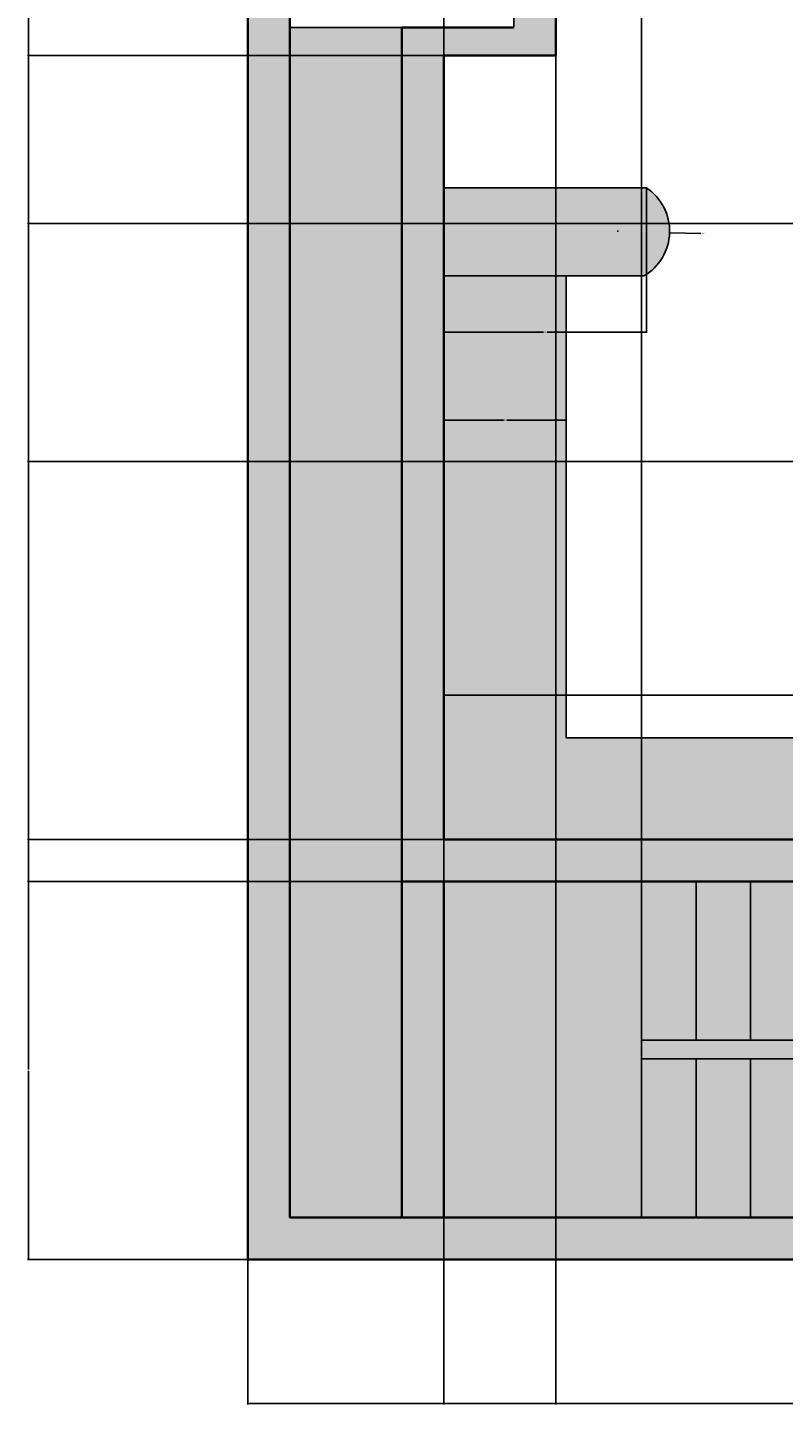
# Model space of a CAD drawing. Units: inches. Extents: x 2549 to 3108, y 1683 to 2362.
# Tile 1 of 30: x 2549 to 2711, y 1683 to 1979. Entities that reach past the tile are written whole.
import ezdxf

# ---------------------------------------------------------------- set-up
doc = ezdxf.new("R2010")
doc.units = ezdxf.units.IN
for name, color, linetype, lineweight in [('A-ANNO-DIMS', 2, 'Continuous', 18), ('A-FLOR', 7, 'Continuous', 25), ('A-FLOR-CASE', 8, 'Continuous', 25), ('A-FLOR-CASE-PATT', 42, 'Continuous', 13), ('A-FLOR-STRS', 7, 'Continuous', 25), ('A-FLOR-STRS-PATT', 41, 'Continuous', 13), ('A-WALL', 7, 'Continuous', 35), ('A-WALL-PATT', 89, 'Continuous', 13), ('C-PROP', 7, 'Continuous', 35)]:
    doc.layers.add(name, color=color, linetype=linetype, lineweight=lineweight)
for name, color, linetype, lineweight, true_color in [('C-PKNG-VEHI-PATT', 251, 'Continuous', 13, 0x636466), ('C-PROP-PATT', 252, 'Continuous', 13, 0x939598), ('C-PVMT-PATT', 9, 'Continuous', 13, 0xc7c8ca)]:
    doc.layers.add(name, color=color, linetype=linetype, lineweight=lineweight, true_color=true_color)
doc.styles.get("Standard").update_dxf_attribs({"font": 'arial.ttf'})
doc.dimstyles.get("Standard").update_dxf_attribs({"dimtxt": 0.18, "dimasz": 0.18, "dimexe": 0.18, "dimexo": 0.0625, "dimgap": 0.09, "dimtad": 0, "dimtih": 1, "dimtoh": 1, "dimdec": 4, "dimzin": 0, "dimdsep": 46, "dimtxsty": 'Standard', "dimcen": 0.09, "dimadec": 0, "dimazin": 0, "dimtfac": 1, "dimtdec": 4, "dimtofl": 0, "dimtmove": 0, "dimatfit": 3, "dimfxl": 1, "dimtolj": 1, "dimtzin": 0, "dimarcsym": 0})

# ---------------------------------------------------------------- blocks, each defined once
blk = doc.blocks.new('*D24')
at = {"layer": 'A-ANNO-DIMS', "color": 0, "lineweight": -2, "transparency": 16777216}
for p, q in [((2596.64, 1714.46), (2596.64, 1683.44)), ((3076.64, 1714.46), (3076.64, 1683.44)), ((2596.82, 1683.62), (2836.35, 1683.62)), ((3076.46, 1683.62), (2836.93, 1683.62))]:
    blk.add_line(p, q, dxfattribs=at)
at = {"layer": 'A-ANNO-DIMS', "color": 0, "transparency": 16777216}
for points in [[(2596.82, 1683.65), (2596.82, 1683.59), (2596.64, 1683.62)], [(3076.46, 1683.65), (3076.46, 1683.59), (3076.64, 1683.62)]]:
    blk.add_solid(points, dxfattribs=at)
at = {"layer": 'Defpoints', "color": 0, "transparency": 16777216}
for p in [(2596.64, 1714.52), (3076.64, 1714.52), (3076.64, 1683.62)]:
    blk.add_point(p, dxfattribs=at)
at = {"layer": 'A-ANNO-DIMS', "color": 0, "transparency": 16777216, "insert": (2836.64, 1683.62), "char_height": 0.18, "attachment_point": 5}
blk.add_mtext('\\A1;480', dxfattribs=at)
blk = doc.blocks.new('*D34')
at = {"layer": 'A-ANNO-DIMS', "color": 0, "lineweight": -2, "transparency": 16777216}
for p, q in [((2629.58, 2074.52), (2549.42, 2074.52)), ((2549.6, 2074.34), (2549.6, 2023.71)), ((2549.6, 1972.7), (2549.6, 2023.34)), ((2638.58, 1972.52), (2549.42, 1972.52))]:
    blk.add_line(p, q, dxfattribs=at)
at = {"layer": 'A-ANNO-DIMS', "color": 0, "transparency": 16777216}
for points in [[(2549.57, 2074.34), (2549.63, 2074.34), (2549.6, 2074.52)], [(2549.57, 1972.7), (2549.63, 1972.7), (2549.6, 1972.52)]]:
    blk.add_solid(points, dxfattribs=at)
at = {"layer": 'Defpoints', "color": 0, "transparency": 16777216}
for p in [(2549.6, 2074.52), (2629.64, 2074.52), (2638.64, 1972.52)]:
    blk.add_point(p, dxfattribs=at)
at = {"layer": 'A-ANNO-DIMS', "color": 0, "transparency": 16777216, "insert": (2549.6, 2023.52), "char_height": 0.18, "attachment_point": 5}
blk.add_mtext('\\A1;102', dxfattribs=at)
blk = doc.blocks.new('*D35')
at = {"layer": 'A-ANNO-DIMS', "color": 0, "lineweight": -2, "transparency": 16777216}
for p, q in [((2638.58, 1972.52), (2549.42, 1972.52)), ((2549.6, 1972.34), (2549.6, 1884.2)), ((2549.6, 1795.7), (2549.6, 1883.84)), ((2629.58, 1795.52), (2549.42, 1795.52))]:
    blk.add_line(p, q, dxfattribs=at)
at = {"layer": 'A-ANNO-DIMS', "color": 0, "transparency": 16777216}
for points in [[(2549.57, 1972.34), (2549.63, 1972.34), (2549.6, 1972.52)], [(2549.57, 1795.7), (2549.63, 1795.7), (2549.6, 1795.52)]]:
    blk.add_solid(points, dxfattribs=at)
at = {"layer": 'Defpoints', "color": 0, "transparency": 16777216}
for p in [(2549.6, 1972.52), (2638.64, 1972.52), (2629.64, 1795.52)]:
    blk.add_point(p, dxfattribs=at)
at = {"layer": 'A-ANNO-DIMS', "color": 0, "transparency": 16777216, "insert": (2549.6, 1884.02), "char_height": 0.18, "attachment_point": 5}
blk.add_mtext('\\A1;177', dxfattribs=at)
blk = doc.blocks.new('*D36')
at = {"layer": 'A-ANNO-DIMS', "color": 0, "lineweight": -2, "transparency": 16777216}
for p, q in [((2629.58, 1795.52), (2549.42, 1795.52)), ((2549.6, 1795.34), (2549.6, 1755.21)), ((2549.6, 1714.7), (2549.6, 1754.84)), ((2596.58, 1714.52), (2549.42, 1714.52))]:
    blk.add_line(p, q, dxfattribs=at)
at = {"layer": 'A-ANNO-DIMS', "color": 0, "transparency": 16777216}
for points in [[(2549.57, 1795.34), (2549.63, 1795.34), (2549.6, 1795.52)], [(2549.57, 1714.7), (2549.63, 1714.7), (2549.6, 1714.52)]]:
    blk.add_solid(points, dxfattribs=at)
at = {"layer": 'Defpoints', "color": 0, "transparency": 16777216}
for p in [(2549.6, 1795.52), (2629.64, 1795.52), (2596.64, 1714.52)]:
    blk.add_point(p, dxfattribs=at)
at = {"layer": 'A-ANNO-DIMS', "color": 0, "transparency": 16777216, "insert": (2549.6, 1755.02), "char_height": 0.18, "attachment_point": 5}
blk.add_mtext('\\A1;81', dxfattribs=at)
blk = doc.blocks.new('*D42')
at = {"layer": 'A-ANNO-DIMS', "color": 0, "lineweight": -2, "transparency": 16777216}
for p, q in [((2638.64, 2080.46), (2638.64, 1683.44)), ((2728.64, 2080.46), (2728.64, 1683.44)), ((2638.82, 1683.62), (2683.42, 1683.62)), ((2728.46, 1683.62), (2683.86, 1683.62))]:
    blk.add_line(p, q, dxfattribs=at)
at = {"layer": 'A-ANNO-DIMS', "color": 0, "transparency": 16777216}
for points in [[(2638.82, 1683.65), (2638.82, 1683.59), (2638.64, 1683.62)], [(2728.46, 1683.65), (2728.46, 1683.59), (2728.64, 1683.62)]]:
    blk.add_solid(points, dxfattribs=at)
at = {"layer": 'Defpoints', "color": 0, "transparency": 16777216}
for p in [(2638.64, 2080.52), (2728.64, 2080.52), (2728.64, 1683.62)]:
    blk.add_point(p, dxfattribs=at)
at = {"layer": 'A-ANNO-DIMS', "color": 0, "transparency": 16777216, "insert": (2683.64, 1683.62), "char_height": 0.18, "attachment_point": 5}
blk.add_mtext('\\A1;90', dxfattribs=at)
blk = doc.blocks.new('*D44')
at = {"layer": 'A-ANNO-DIMS', "color": 0, "lineweight": -2, "transparency": 16777216}
for p, q in [((2662.64, 2040.99), (2662.64, 1683.44)), ((2806.64, 2016.13), (2806.64, 1683.44)), ((2662.82, 1683.62), (2734.36, 1683.62)), ((2806.46, 1683.62), (2734.92, 1683.62))]:
    blk.add_line(p, q, dxfattribs=at)
at = {"layer": 'A-ANNO-DIMS', "color": 0, "transparency": 16777216}
for points in [[(2662.82, 1683.65), (2662.82, 1683.59), (2662.64, 1683.62)], [(2806.46, 1683.65), (2806.46, 1683.59), (2806.64, 1683.62)]]:
    blk.add_solid(points, dxfattribs=at)
at = {"layer": 'Defpoints', "color": 0, "transparency": 16777216}
for p in [(2662.64, 2041.06), (2806.64, 2016.19), (2806.64, 1683.62)]:
    blk.add_point(p, dxfattribs=at)
at = {"layer": 'A-ANNO-DIMS', "color": 0, "transparency": 16777216, "insert": (2734.64, 1683.62), "char_height": 0.18, "attachment_point": 5}
blk.add_mtext('\\A1;144', dxfattribs=at)
blk = doc.blocks.new('*D45')
at = {"layer": 'A-ANNO-DIMS', "color": 0, "lineweight": -2, "transparency": 16777216}
for p, q in [((2605.64, 1978.59), (2605.64, 2009.6)), ((2653.64, 1978.59), (2653.64, 2009.6)), ((2605.82, 2009.42), (2629.42, 2009.42)), ((2653.46, 2009.42), (2629.87, 2009.42))]:
    blk.add_line(p, q, dxfattribs=at)
at = {"layer": 'A-ANNO-DIMS', "color": 0, "transparency": 16777216}
for points in [[(2605.82, 2009.45), (2605.82, 2009.39), (2605.64, 2009.42)], [(2653.46, 2009.45), (2653.46, 2009.39), (2653.64, 2009.42)]]:
    blk.add_solid(points, dxfattribs=at)
at = {"layer": 'Defpoints', "color": 0, "transparency": 16777216}
for p in [(2653.64, 2009.42), (2605.64, 1978.52), (2653.64, 1978.52)]:
    blk.add_point(p, dxfattribs=at)
at = {"layer": 'A-ANNO-DIMS', "color": 0, "transparency": 16777216, "insert": (2629.64, 2009.42), "char_height": 0.18, "attachment_point": 5}
blk.add_mtext('\\A1;48', dxfattribs=at)
blk = doc.blocks.new('*D49')
at = {"layer": 'A-ANNO-DIMS', "color": 0, "lineweight": -2, "transparency": 16777216}
for p, q in [((2638.64, 1804.59), (2638.64, 1835.6)), ((2638.82, 1835.42), (2722.36, 1835.42)), ((2806.46, 1835.42), (2722.92, 1835.42)), ((2806.64, 1804.59), (2806.64, 1835.6))]:
    blk.add_line(p, q, dxfattribs=at)
at = {"layer": 'A-ANNO-DIMS', "color": 0, "transparency": 16777216}
for points in [[(2638.82, 1835.45), (2638.82, 1835.39), (2638.64, 1835.42)], [(2806.46, 1835.45), (2806.46, 1835.39), (2806.64, 1835.42)]]:
    blk.add_solid(points, dxfattribs=at)
at = {"layer": 'Defpoints', "color": 0, "transparency": 16777216}
for p in [(2806.64, 1835.42), (2638.64, 1804.52), (2806.64, 1804.52)]:
    blk.add_point(p, dxfattribs=at)
at = {"layer": 'A-ANNO-DIMS', "color": 0, "transparency": 16777216, "insert": (2722.64, 1835.42), "char_height": 0.18, "attachment_point": 5}
blk.add_mtext('\\A1;168', dxfattribs=at)
blk = doc.blocks.new('*D50')
at = {"layer": 'A-ANNO-DIMS', "color": 0, "lineweight": -2, "transparency": 16777216}
for p, q in [((2638.64, 1944.09), (2638.64, 1913.07)), ((2682.05, 1944.09), (2682.05, 1913.07)), ((2638.82, 1913.25), (2659.97, 1913.25)), ((2681.87, 1913.25), (2660.73, 1913.25))]:
    blk.add_line(p, q, dxfattribs=at)
at = {"layer": 'A-ANNO-DIMS', "color": 0, "transparency": 16777216}
for points in [[(2638.82, 1913.28), (2638.82, 1913.22), (2638.64, 1913.25)], [(2681.87, 1913.28), (2681.87, 1913.22), (2682.05, 1913.25)]]:
    blk.add_solid(points, dxfattribs=at)
at = {"layer": 'Defpoints', "color": 0, "transparency": 16777216}
for p in [(2638.64, 1944.15), (2682.05, 1944.15), (2638.64, 1913.25)]:
    blk.add_point(p, dxfattribs=at)
at = {"layer": 'A-ANNO-DIMS', "color": 0, "transparency": 16777216, "insert": (2660.35, 1913.25), "char_height": 0.18, "attachment_point": 5}
blk.add_mtext('\\A1;43.41', dxfattribs=at)
blk = doc.blocks.new('*D51')
at = {"layer": 'A-ANNO-DIMS', "color": 0, "lineweight": -2, "transparency": 16777216}
for p, q in [((2638.64, 1925.23), (2638.64, 1894.21)), ((2664.85, 1925.23), (2664.85, 1894.21)), ((2638.82, 1894.39), (2651.37, 1894.39)), ((2664.67, 1894.39), (2652.13, 1894.39))]:
    blk.add_line(p, q, dxfattribs=at)
at = {"layer": 'A-ANNO-DIMS', "color": 0, "transparency": 16777216}
for points in [[(2638.82, 1894.42), (2638.82, 1894.36), (2638.64, 1894.39)], [(2664.67, 1894.42), (2664.67, 1894.36), (2664.85, 1894.39)]]:
    blk.add_solid(points, dxfattribs=at)
at = {"layer": 'Defpoints', "color": 0, "transparency": 16777216}
for p in [(2638.64, 1925.29), (2664.85, 1925.29), (2638.64, 1894.39)]:
    blk.add_point(p, dxfattribs=at)
at = {"layer": 'A-ANNO-DIMS', "color": 0, "transparency": 16777216, "insert": (2651.75, 1894.39), "char_height": 0.18, "attachment_point": 5}
blk.add_mtext('\\A1;26.21', dxfattribs=at)
blk = doc.blocks.new('*D55')
at = {"layer": 'A-ANNO-DIMS', "color": 0, "lineweight": -2, "transparency": 16777216}
for p, q in [((2872.58, 1885.52), (2549.42, 1885.52)), ((2549.6, 1885.34), (2549.6, 1845.21)), ((2549.6, 1804.7), (2549.6, 1844.84)), ((2872.58, 1804.52), (2549.42, 1804.52))]:
    blk.add_line(p, q, dxfattribs=at)
at = {"layer": 'A-ANNO-DIMS', "color": 0, "transparency": 16777216}
for points in [[(2549.57, 1885.34), (2549.63, 1885.34), (2549.6, 1885.52)], [(2549.57, 1804.7), (2549.63, 1804.7), (2549.6, 1804.52)]]:
    blk.add_solid(points, dxfattribs=at)
at = {"layer": 'Defpoints', "color": 0, "transparency": 16777216}
for p in [(2549.6, 1885.52), (2872.64, 1885.52), (2872.64, 1804.52)]:
    blk.add_point(p, dxfattribs=at)
at = {"layer": 'A-ANNO-DIMS', "color": 0, "transparency": 16777216, "insert": (2549.6, 1845.02), "char_height": 0.18, "attachment_point": 5}
blk.add_mtext('\\A1;81', dxfattribs=at)
blk = doc.blocks.new('*D56')
at = {"layer": 'A-ANNO-DIMS', "color": 0, "lineweight": -2, "transparency": 16777216}
for p, q in [((3043.58, 1936.52), (2549.42, 1936.52)), ((2549.6, 1936.34), (2549.6, 1911.21)), ((2549.6, 1885.7), (2549.6, 1910.84)), ((3043.58, 1885.52), (2549.42, 1885.52))]:
    blk.add_line(p, q, dxfattribs=at)
at = {"layer": 'A-ANNO-DIMS', "color": 0, "transparency": 16777216}
for points in [[(2549.57, 1936.34), (2549.63, 1936.34), (2549.6, 1936.52)], [(2549.57, 1885.7), (2549.63, 1885.7), (2549.6, 1885.52)]]:
    blk.add_solid(points, dxfattribs=at)
at = {"layer": 'Defpoints', "color": 0, "transparency": 16777216}
for p in [(2549.6, 1936.52), (3043.64, 1936.52), (3043.64, 1885.52)]:
    blk.add_point(p, dxfattribs=at)
at = {"layer": 'A-ANNO-DIMS', "color": 0, "transparency": 16777216, "insert": (2549.6, 1911.02), "char_height": 0.18, "attachment_point": 5}
blk.add_mtext('\\A1;51', dxfattribs=at)
blk = doc.blocks.new('*D59')
at = {"layer": 'A-ANNO-DIMS', "color": 0, "lineweight": -2, "transparency": 16777216}
for p, q in [((2680.98, 1761.59), (2680.98, 2362.32)), ((2681.16, 2362.14), (2733.11, 2362.14)), ((2785.98, 2362.14), (2734.02, 2362.14)), ((2786.16, 1761.59), (2786.16, 2362.32))]:
    blk.add_line(p, q, dxfattribs=at)
at = {"layer": 'A-ANNO-DIMS', "color": 0, "transparency": 16777216}
for points in [[(2681.16, 2362.17), (2681.16, 2362.11), (2680.98, 2362.14)], [(2785.98, 2362.17), (2785.98, 2362.11), (2786.16, 2362.14)]]:
    blk.add_solid(points, dxfattribs=at)
at = {"layer": 'Defpoints', "color": 0, "transparency": 16777216}
for p in [(2786.16, 2362.14), (2680.98, 1761.52), (2786.16, 1761.52)]:
    blk.add_point(p, dxfattribs=at)
at = {"layer": 'A-ANNO-DIMS', "color": 0, "transparency": 16777216, "insert": (2733.57, 2362.14), "char_height": 0.18, "attachment_point": 5}
blk.add_mtext('\\A1;105.18', dxfattribs=at)
blk = doc.blocks.new('*D62')
at = {"layer": 'A-ANNO-DIMS', "color": 0, "lineweight": -2, "transparency": 16777216}
for p, q in [((2675.78, 1934.89), (2675.96, 1934.89)), ((2675.87, 1934.8), (2675.87, 1934.98)), ((2693.67, 1934.38), (2687.18, 1934.56))]:
    blk.add_line(p, q, dxfattribs=at)
at = {"layer": 'A-ANNO-DIMS', "color": 0, "transparency": 16777216}
blk.add_solid([(2687.18, 1934.59), (2687.18, 1934.53), (2687, 1934.57)], dxfattribs=at)
at = {"layer": 'Defpoints', "color": 0, "transparency": 16777216}
for p in [(2675.87, 1934.89), (2687, 1934.57)]:
    blk.add_point(p, dxfattribs=at)
at = {"layer": 'A-ANNO-DIMS', "color": 0, "transparency": 16777216, "insert": (2694.15, 1934.38), "char_height": 0.18, "attachment_point": 5}
blk.add_mtext('\\A1;R11.13', dxfattribs=at)

msp = doc.modelspace()

# ---------------------------------------------------------------- hatches: boundary and pattern name
at = {"layer": 'A-FLOR-CASE-PATT', "transparency": 33554595}
h = msp.add_hatch(color=256, dxfattribs=at)
h.dxf.hatch_style = 1
h.paths.add_polyline_path([(2682.0533, 1944.149), (2638.6427, 1944.149), (2638.6427, 1925.2912), (2681.5046, 1925.2912, 0.55362962)])
at = {"layer": 'A-FLOR-CASE-PATT', "transparency": 33554539}
h = msp.add_hatch(color=256, dxfattribs=at)
h.dxf.hatch_style = 1
h.paths.add_polyline_path([(2664.8522, 1925.2912), (2638.6427, 1925.2912), (2638.6427, 1804.5237), (2662.6427, 1804.5237), (2806.6427, 1804.5237), (2806.6427, 1826.2821), (2664.8522, 1826.2821)])
h.paths.add_polyline_path([(2872.6427, 1885.5237), (2858.0172, 1885.5237), (2858.0172, 1818.9517), (2812.6427, 1818.9517), (2812.6427, 1804.5237), (2872.6427, 1804.5237)])
at = {"layer": 'A-FLOR-STRS-PATT', "transparency": 33554567}
h = msp.add_hatch(color=256, dxfattribs=at)
h.dxf.hatch_style = 1
h.paths.add_polyline_path([(2680.9778, 1795.5237), (2662.6427, 1795.5237), (2638.6427, 1795.5237), (2638.6427, 1723.5237), (2680.9778, 1723.5237)])
h.paths.add_polyline_path([(2692.6645, 1795.5237), (2680.9778, 1795.5237), (2680.9778, 1761.5237), (2692.6645, 1761.5237)])
h.paths.add_polyline_path([(2704.3511, 1795.5237), (2692.6645, 1795.5237), (2692.6645, 1761.5237), (2704.3511, 1761.5237)])
h.paths.add_polyline_path([(2716.0378, 1795.5237), (2704.3511, 1795.5237), (2704.3511, 1761.5237), (2716.0378, 1761.5237)])
h.paths.add_polyline_path([(2727.7244, 1795.5237), (2716.0378, 1795.5237), (2716.0378, 1761.5237), (2727.7244, 1761.5237)])
h.paths.add_polyline_path([(2739.4111, 1795.5237), (2727.7244, 1795.5237), (2727.7244, 1761.5237), (2739.4111, 1761.5237)])
h.paths.add_polyline_path([(2751.0977, 1795.5237), (2739.4111, 1795.5237), (2739.4111, 1761.5237), (2751.0977, 1761.5237)])
h.paths.add_polyline_path([(2786.1577, 1757.5237), (2774.471, 1757.5237), (2774.471, 1723.5237), (2786.1577, 1723.5237)])
h.paths.add_polyline_path([(2774.471, 1757.5237), (2762.7844, 1757.5237), (2762.7844, 1723.5237), (2774.471, 1723.5237)])
h.paths.add_polyline_path([(2762.7844, 1757.5237), (2751.0977, 1757.5237), (2751.0977, 1723.5237), (2762.7844, 1723.5237)])
h.paths.add_polyline_path([(2751.0977, 1757.5237), (2739.4111, 1757.5237), (2739.4111, 1723.5237), (2751.0977, 1723.5237)])
h.paths.add_polyline_path([(2727.7244, 1757.5237), (2716.0378, 1757.5237), (2716.0378, 1723.5237), (2727.7244, 1723.5237)])
h.paths.add_polyline_path([(2716.0378, 1757.5237), (2704.3511, 1757.5237), (2704.3511, 1723.5237), (2716.0378, 1723.5237)])
h.paths.add_polyline_path([(2704.3511, 1757.5237), (2692.6645, 1757.5237), (2692.6645, 1723.5237), (2704.3511, 1723.5237)])
h.paths.add_polyline_path([(2692.6645, 1757.5237), (2680.9778, 1757.5237), (2680.9778, 1723.5237), (2692.6645, 1723.5237)])
h.paths.add_polyline_path([(2739.4111, 1757.5237), (2727.7244, 1757.5237), (2727.7244, 1723.5237), (2739.4111, 1723.5237)])
h.paths.add_polyline_path([(2786.1577, 1761.5237), (2680.9778, 1761.5237), (2680.9778, 1757.5237), (2786.1577, 1757.5237)])
at = {"layer": 'A-WALL-PATT'}
h = msp.add_hatch(color=256, dxfattribs=at)
h.dxf.hatch_style = 1
h.paths.add_polyline_path([(2638.6427, 2272.5237), (3034.6427, 2272.5237), (3034.6427, 1936.5237), (3043.6427, 1936.5237), (3043.6427, 2281.5237), (2629.6427, 2281.5237), (2629.6427, 2074.5237), (2812.6427, 2074.5237), (2812.6427, 2140.5237), (2785.7177, 2140.5237), (2785.7177, 2134.5237), (2806.6427, 2134.5237), (2806.6427, 2080.5237), (2638.6427, 2080.5237)])
h.paths.add_polyline_path([(2638.6427, 1972.5237), (2662.6427, 1972.5237), (2662.6427, 2041.0557), (2653.6427, 2041.0557), (2653.6427, 1978.5237), (2629.6427, 1978.5237), (2629.6427, 1795.5237), (2662.6427, 1795.5237), (2881.6427, 1795.5237), (2881.6427, 1936.5237), (2965.9351, 1936.5237), (2965.9351, 1974.5439), (2959.9351, 1974.5439), (2959.9351, 1945.5237), (2881.6427, 1945.5237), (2872.6427, 1945.5237), (2872.6427, 1804.5237), (2662.6427, 1804.5237), (2638.6427, 1804.5237)])
h = msp.add_hatch(color=256, dxfattribs=at)
h.dxf.hatch_style = 1
h.paths.add_polyline_path([(2638.6427, 1795.5237), (2629.6427, 1795.5237), (2629.6427, 1723.5237), (2638.6427, 1723.5237)])
at = {"layer": 'C-PKNG-VEHI-PATT'}
h = msp.add_hatch(color=256, dxfattribs=at)
h.dxf.hatch_style = 1
edge = h.paths.add_edge_path()
edge.add_ellipse((2935.7258, 1791.964), major_axis=(-50.66, 0), ratio=0.84230387, start_angle=248.165046, end_angle=265.722579)
edge.add_line((2938.911, 1834.5507), (2925.8653, 1834.5507))
edge.add_ellipse((2929.0505, 1791.964), major_axis=(50.66, 0), ratio=0.84230387, start_angle=94.277421, end_angle=111.834954)
edge.add_line((2912.8508, 1832.3947), (2914.2044, 1822.2495))
edge.add_ellipse((2930.6538, 1783.1023), major_axis=(-49.3014, 0), ratio=0.84230387, start_angle=-85.12993, end_angle=-67.208085, ccw=False)
edge.add_line((2927.1247, 1824.5225), (2937.6516, 1824.5225))
edge.add_ellipse((2934.1225, 1783.1023), major_axis=(49.3014, 0), ratio=0.84230387, start_angle=67.208085, end_angle=85.12993, ccw=False)
edge.add_line((2950.5719, 1822.2495), (2951.9255, 1832.3947))
edge = h.paths.add_edge_path()
edge.add_ellipse((2903.4793, 1857.3351), major_axis=(-34.7979, 0), ratio=0.84230387, start_angle=180, end_angle=209.43857)
edge.add_ellipse((2961.297, 1857.3351), major_axis=(34.7979, 0), ratio=0.84230387, start_angle=150.56143, end_angle=180)
edge.add_line((2926.4991, 1857.3351), (2926.4991, 1843.7609))
edge.add_ellipse((2924.1251, 1844.3143), major_axis=(-0.2209, 3.9278), ratio=0.60383358, start_angle=89.002014, end_angle=253.657408, ccw=False)
edge.add_line((2921.7512, 1844.2222), (2921.7512, 1853.3975))
edge.add_line((2921.7512, 1853.3975), (2925.269, 1855.8484))
edge.add_ellipse((2925.4782, 1855.4931), major_axis=(0.4584, 0), ratio=0.84230387, start_angle=90, end_angle=134.480211, ccw=False)
edge.add_line((2925.4782, 1855.8792), (2926.4991, 1855.8792))
edge.add_line((2926.4991, 1855.8792), (2926.4991, 1857.3351))
edge.add_ellipse((2961.297, 1857.3351), major_axis=(34.7979, 0), ratio=0.84230387, start_angle=150.56143, end_angle=180, ccw=False)
edge.add_line((2932.3882, 1873.6501), (2932.3882, 1875.7801))
edge.add_ellipse((2932.3882, 1875.3939), major_axis=(0.4584, 0), ratio=0.84230387, start_angle=90, end_angle=127.93313)
edge.add_line((2932.1366, 1875.7167), (2928.5915, 1873.7564))
edge.add_ellipse((2899.9271, 2002.4692), major_axis=(155.4756, 0), ratio=0.84230387, start_angle=-80.743434, end_angle=-77.445067, ccw=False)
edge.add_ellipse((2949.4402, 1715.2151), major_axis=(-189.1422, 0), ratio=0.84230387, start_angle=-79.790461, end_angle=-77.555373)
edge.add_ellipse((3300.3614, 1852.5642), major_axis=(-386.1662, 0), ratio=0.84230387, start_angle=-2.863715, end_angle=2.198541)
edge.add_ellipse((2929.0505, 1792.5159), major_axis=(-55.6192, 0), ratio=0.84230387, start_angle=-85.917589, end_angle=-72.280047, ccw=False)
edge.add_line((2925.7129, 1839.2798), (2939.0634, 1839.2798))
edge.add_ellipse((2935.7258, 1792.5159), major_axis=(55.6192, 0), ratio=0.84230387, start_angle=72.280047, end_angle=85.917589, ccw=False)
edge.add_ellipse((2564.4149, 1852.5642), major_axis=(-386.1662, 0), ratio=0.84230387, start_angle=177.801459, end_angle=182.863715)
edge.add_ellipse((2915.3361, 1715.2151), major_axis=(189.1422, 0), ratio=0.84230387, start_angle=77.555373, end_angle=79.790461)
edge.add_ellipse((2964.8492, 2002.4692), major_axis=(-155.4756, 0), ratio=0.84230387, start_angle=77.445067, end_angle=80.743434, ccw=False)
edge.add_line((2936.1848, 1873.7564), (2932.6397, 1875.7167))
edge.add_ellipse((2932.3882, 1875.3939), major_axis=(0.4584, 0), ratio=0.84230387, start_angle=52.06687, end_angle=90)
edge.add_line((2932.3882, 1875.7801), (2932.3882, 1873.6501))
edge.add_ellipse((2903.4793, 1857.3351), major_axis=(-34.7979, 0), ratio=0.84230387, start_angle=180, end_angle=209.43857, ccw=False)
edge.add_line((2938.2772, 1857.3351), (2938.2772, 1855.8792))
edge.add_line((2938.2772, 1855.8792), (2939.4059, 1855.8792))
edge.add_ellipse((2939.2981, 1855.4931), major_axis=(-0.4584, 0), ratio=0.84230387, start_angle=225.519789, end_angle=270, ccw=False)
edge.add_line((2939.5903, 1855.7906), (2943.0251, 1853.3975))
edge.add_line((2943.0251, 1853.3975), (2943.0251, 1844.2222))
edge.add_ellipse((2940.6512, 1844.3143), major_axis=(0.2209, 3.9278), ratio=0.60383358, start_angle=106.342592, end_angle=270.997986, ccw=False)
edge.add_line((2938.2772, 1843.7609), (2938.2772, 1857.3351))
edge = h.paths.add_edge_path()
edge.add_ellipse((2932.3882, 1865.1973), major_axis=(91.081, 0), ratio=0.84230387, start_angle=256.401865, end_angle=283.598135, ccw=False)
edge.add_line((2914.2044, 1790.0239), (2914.2044, 1778.3622))
edge.add_ellipse((2932.3882, 1853.5356), major_axis=(91.081, 0), ratio=0.84230387, start_angle=256.401865, end_angle=283.598135)
edge.add_line((2950.5719, 1778.3622), (2950.5719, 1790.0239))
edge = h.paths.add_edge_path()
edge.add_ellipse((2948.7383, 1772.3145), major_axis=(1.8336, 0), ratio=0.84230387, start_angle=0, end_angle=90)
edge.add_line((2948.7383, 1773.859), (2916.038, 1773.859))
edge.add_ellipse((2916.038, 1772.3145), major_axis=(1.8336, 0), ratio=0.84230387, start_angle=90, end_angle=180)
edge.add_line((2914.2044, 1772.3145), (2914.2044, 1760.2558))
edge.add_line((2914.2044, 1760.2558), (2950.5719, 1760.2558))
edge.add_line((2950.5719, 1760.2558), (2950.5719, 1772.3145))
h.paths.add_polyline_path([(2748.8496, 2101.6383), (2798.148, 2101.6383), (2798.148, 2111.4248), (2748.8496, 2111.4248)], flags=9)
h.paths.add_polyline_path([(2685.2081, 2101.489), (2719.3253, 2101.489), (2719.3253, 2111.2819), (2685.2081, 2111.2819)], flags=9)
h.paths.add_polyline_path([(2814.6852, 1907.1328), (2847.8384, 1907.1328), (2847.8384, 1916.9258), (2814.6852, 1916.9258)], flags=9)
h.paths.add_polyline_path([(2814.3906, 1835.5864), (2848.0172, 1835.5864), (2848.0172, 1845.3794), (2814.3906, 1845.3794)], flags=9)
h.paths.add_polyline_path([(2800.5245, 1759.1674), (2853.7435, 1759.1674), (2853.7435, 1768.954), (2800.5245, 1768.954)], flags=9)
h.paths.add_polyline_path([(2972.4611, 1807.3305), (3015.3943, 1807.3305), (3015.3943, 1817.117), (2972.4611, 1817.117)], flags=9)
h.paths.add_polyline_path([(2902.3327, 1888.6731), (2937.9131, 1888.6731), (2937.9131, 1898.4661), (2902.3327, 1898.4661)], flags=9)
h.paths.add_polyline_path([(2712.1779, 1878.9039), (2754.1257, 1878.9039), (2754.1257, 1888.6904), (2712.1779, 1888.6904)], flags=9)
h.paths.add_polyline_path([(2614.0056, 2012.812), (2650.0251, 2012.812), (2650.0251, 2022.4371), (2614.0056, 2022.4371)], flags=9)
h.paths.add_polyline_path([(2713.3129, 2003.1645), (2747.4237, 2003.1645), (2747.4237, 2012.951), (2713.3129, 2012.951)], flags=9)
h.paths.add_polyline_path([(2950.1379, 2001.6934), (2982.2992, 2001.6934), (2982.2992, 2011.48), (2950.1379, 2011.48)], flags=9)
h.paths.add_polyline_path([(2940.864, 2238.5537), (2997.5066, 2238.5537), (2997.5066, 2248.3466), (2940.864, 2248.3466)], flags=9)
h.paths.add_polyline_path([(2821.5457, 2202.8348), (2855.663, 2202.8348), (2855.663, 2212.6278), (2821.5457, 2212.6278)], flags=9)
h.paths.add_polyline_path([(2661.8026, 2238.6249), (2718.4451, 2238.6249), (2718.4451, 2248.4179), (2661.8026, 2248.4179)], flags=9)
at = {"layer": 'C-PROP-PATT'}
h = msp.add_hatch(color=256, dxfattribs=at)
h.dxf.hatch_style = 1
h.paths.add_polyline_path([(3076.6427, 2314.5237), (2596.6427, 2314.5237), (2596.6427, 1714.5237), (2881.84, 1714.5237), (2881.84, 1723.5237), (2605.6427, 1723.5237), (2605.6427, 2305.5237), (3067.6427, 2305.5237), (3067.6427, 1723.5237), (3067.6427, 1714.5237), (3076.6427, 1714.5237)])
at = {"layer": 'C-PVMT-PATT'}
h = msp.add_hatch(color=256, dxfattribs=at)
h.dxf.hatch_style = 1
h.paths.add_polyline_path([(3067.6427, 2305.5237), (2605.6427, 2305.5237), (2605.6427, 2074.5237), (2629.6427, 2074.5237), (2629.6427, 2281.5237), (3043.6427, 2281.5237), (3043.6427, 1885.5237), (3043.6427, 1872.8745), (3031.1672, 1872.8745), (3031.1672, 1862.5731), (2995.8054, 1862.5731), (2995.8054, 1872.8745), (2983.1752, 1872.8745), (2983.1752, 1885.5237), (2881.6427, 1885.5237), (2881.6427, 1795.5237), (2751.0977, 1795.5237), (2751.0977, 1761.5237), (2786.1577, 1761.5237), (2786.1577, 1723.5237), (2881.84, 1723.5237), (2881.84, 1714.5237), (3067.6427, 1714.5237), (3067.6427, 1723.5237)])
edge = h.paths.add_edge_path(flags=16)
edge.add_ellipse((2949.4402, 1710.9683), major_axis=(-194.1014, 0), ratio=0.84230387, start_angle=-77.874034, end_angle=-76.219471, ccw=False)
edge.add_ellipse((2949.4402, 1715.2151), major_axis=(-189.1422, 0), ratio=0.84230387, start_angle=-79.790461, end_angle=-77.555373, ccw=False)
edge.add_ellipse((2899.9271, 2002.4692), major_axis=(155.4756, 0), ratio=0.84230387, start_angle=-80.743434, end_angle=-77.445067)
edge.add_line((2928.5915, 1873.7564), (2932.3882, 1875.8558))
edge.add_line((2932.3882, 1875.8558), (2936.1848, 1873.7564))
edge.add_ellipse((2964.8492, 2002.4692), major_axis=(-155.4756, 0), ratio=0.84230387, start_angle=77.445067, end_angle=80.743434)
edge.add_ellipse((2915.3361, 1715.2151), major_axis=(189.1422, 0), ratio=0.84230387, start_angle=77.555373, end_angle=79.790461, ccw=False)
edge.add_ellipse((2915.3361, 1710.9683), major_axis=(-194.1014, 0), ratio=0.84230387, start_angle=256.219471, end_angle=257.874034, ccw=False)
edge.add_ellipse((2628.2871, 1850.2612), major_axis=(-327.2532, 0), ratio=0.84230387, start_angle=182.17995, end_angle=183.650428, ccw=False)
edge.add_ellipse((2955.5637, 1861.9334), major_axis=(-0.9168, 0), ratio=0.84230387, start_angle=180, end_angle=270, ccw=False)
edge.add_line((2956.4805, 1862.3857), (2956.4805, 1846.4866))
edge.add_ellipse((2955.5637, 1846.939), major_axis=(-0.9168, 0), ratio=0.84230387, start_angle=90, end_angle=180, ccw=False)
edge.add_ellipse((-3607.0606, 1835.832), major_axis=(-6562.6242, 0), ratio=0.84230387, start_angle=179.61613322, end_angle=180.09022909, ccw=False)
edge.add_ellipse((2955.5637, 1791.0926), major_axis=(0.9168, 0), ratio=0.84230387, start_angle=0, end_angle=90, ccw=False)
edge.add_line((2956.4805, 1791.545), (2956.4805, 1775.6459))
edge.add_ellipse((2955.5637, 1776.0982), major_axis=(0.9168, 0), ratio=0.84230387, start_angle=270, end_angle=360, ccw=False)
edge.add_ellipse((-3607.0606, 1835.832), major_axis=(-6562.6242, 0), ratio=0.84230387, start_angle=179.3813568, end_angle=179.47172853, ccw=False)
edge.add_ellipse((2954.5907, 1763.8768), major_axis=(-1.3752, 0), ratio=0.84230387, start_angle=179.371763, end_angle=248.464757, ccw=False)
edge.add_ellipse((-3607.519, 1835.832), major_axis=(-6564.0409, 0), ratio=0.842303863, start_angle=179.35344594, end_angle=179.37176282, ccw=False)
edge.add_ellipse((2952.6829, 1761.8002), major_axis=(3.2503, 0), ratio=0.84230387, start_angle=-90, end_angle=-0.646554, ccw=False)
edge.add_line((2952.6829, 1759.0625), (2912.0934, 1759.0625))
edge.add_ellipse((2912.0934, 1761.8002), major_axis=(3.2503, 0), ratio=0.84230387, start_angle=180.646554, end_angle=270, ccw=False)
edge.add_ellipse((9472.2953, 1835.832), major_axis=(-6564.0409, 0), ratio=0.842303871, start_angle=0.62823722, end_angle=0.6465541, ccw=False)
edge.add_ellipse((2910.1856, 1763.8768), major_axis=(1.3752, 0), ratio=0.84230387, start_angle=111.535244, end_angle=180.628237, ccw=False)
edge.add_ellipse((9471.8369, 1835.832), major_axis=(-6562.6242, 0), ratio=0.84230387, start_angle=0.52827147, end_angle=0.6465541, ccw=False)
edge.add_ellipse((2909.2126, 1776.0982), major_axis=(-0.9168, 0), ratio=0.84230387, start_angle=0, end_angle=90, ccw=False)
edge.add_line((2908.2958, 1775.6459), (2908.2958, 1791.545))
edge.add_ellipse((2909.2126, 1791.0926), major_axis=(-0.9168, 0), ratio=0.84230387, start_angle=-90, end_angle=0, ccw=False)
edge.add_ellipse((9471.8369, 1835.832), major_axis=(-6562.6242, 0), ratio=0.84230387, start_angle=-0.09022909, end_angle=0.38386678, ccw=False)
edge.add_ellipse((2909.2126, 1846.939), major_axis=(-0.9168, 0), ratio=0.84230387, start_angle=0, end_angle=90, ccw=False)
edge.add_line((2908.2958, 1846.4866), (2908.2958, 1862.3857))
edge.add_ellipse((2909.2126, 1861.9334), major_axis=(0.9168, 0), ratio=0.84230387, start_angle=90, end_angle=180, ccw=False)
edge.add_ellipse((3236.4892, 1850.2612), major_axis=(327.2532, 0), ratio=0.84230387, start_angle=176.349572, end_angle=177.82005, ccw=False)
edge = h.paths.add_edge_path(flags=0)
edge.add_ellipse((2903.4793, 1857.3351), major_axis=(-34.7979, 0), ratio=0.84230387, start_angle=180, end_angle=209.43857, ccw=False)
edge.add_line((2938.2772, 1857.3351), (2938.2772, 1855.8792))
edge.add_line((2938.2772, 1855.8792), (2939.4631, 1855.8792))
edge.add_line((2939.4631, 1855.8792), (2943.0251, 1853.3975))
edge.add_line((2943.0251, 1853.3975), (2943.0251, 1844.2222))
edge.add_ellipse((2940.6512, 1844.3143), major_axis=(0.2209, 3.9278), ratio=0.60383358, start_angle=106.342592, end_angle=270.997986, ccw=False)
edge.add_line((2938.2772, 1843.7609), (2938.2772, 1857.3351))
edge.add_ellipse((2903.4793, 1857.3351), major_axis=(-34.7979, 0), ratio=0.84230387, start_angle=180, end_angle=209.43857)
edge.add_ellipse((2961.297, 1857.3351), major_axis=(34.7979, 0), ratio=0.84230387, start_angle=150.56143, end_angle=180)
edge.add_line((2926.4991, 1857.3351), (2926.4991, 1843.7609))
edge.add_ellipse((2924.1251, 1844.3143), major_axis=(-0.2209, 3.9278), ratio=0.60383358, start_angle=89.002014, end_angle=253.657408, ccw=False)
edge.add_line((2921.7512, 1844.2222), (2921.7512, 1853.3975))
edge.add_line((2921.7512, 1853.3975), (2925.3132, 1855.8792))
edge.add_line((2925.3132, 1855.8792), (2926.4991, 1855.8792))
edge.add_line((2926.4991, 1855.8792), (2926.4991, 1857.3351))
edge.add_ellipse((2961.297, 1857.3351), major_axis=(34.7979, 0), ratio=0.84230387, start_angle=150.56143, end_angle=180, ccw=False)
edge = h.paths.add_edge_path(flags=0)
edge.add_ellipse((2929.0505, 1791.964), major_axis=(50.66, 0), ratio=0.84230387, start_angle=94.277421, end_angle=111.834954, ccw=False)
edge.add_line((2925.8653, 1834.5507), (2938.911, 1834.5507))
edge.add_ellipse((2935.7258, 1791.964), major_axis=(-50.66, 0), ratio=0.84230387, start_angle=248.165046, end_angle=265.722579, ccw=False)
edge.add_line((2951.9255, 1832.3947), (2950.5719, 1822.2495))
edge.add_ellipse((2934.1225, 1783.1023), major_axis=(49.3014, 0), ratio=0.84230387, start_angle=67.208085, end_angle=85.12993)
edge.add_line((2937.6516, 1824.5225), (2927.1247, 1824.5225))
edge.add_ellipse((2930.6538, 1783.1023), major_axis=(-49.3014, 0), ratio=0.84230387, start_angle=-85.12993, end_angle=-67.208085)
edge.add_line((2914.2044, 1822.2495), (2912.8508, 1832.3947))
edge = h.paths.add_edge_path(flags=0)
edge.add_line((2910.1338, 1829.4651), (2912.6432, 1821.2711))
edge.add_ellipse((5203.7787, 1816.4367), major_axis=(-2291.1426, 0), ratio=0.84230387, start_angle=-0.1208974, end_angle=0.3640763)
edge.add_line((2912.7012, 1801.8782), (2910.3305, 1792.5698))
edge.add_ellipse((9471.8369, 1835.832), major_axis=(-6561.7074, 0), ratio=0.84230387, start_angle=0.05559431, end_angle=0.37776419, ccw=False)
edge = h.paths.add_edge_path(flags=0)
edge.add_ellipse((-3607.0606, 1835.832), major_axis=(6561.7074, 0), ratio=0.84230387, start_angle=-0.37776419, end_angle=-0.05559431, ccw=False)
edge.add_line((2954.4458, 1792.5698), (2952.0751, 1801.8782))
edge.add_ellipse((660.9976, 1816.4367), major_axis=(2291.1426, 0), ratio=0.84230387, start_angle=-0.3640763, end_angle=0.1208974)
edge.add_line((2952.1331, 1821.2711), (2954.6425, 1829.4651))
edge = h.paths.add_edge_path(flags=0)
edge.add_ellipse((2932.3882, 1865.1973), major_axis=(91.081, 0), ratio=0.84230387, start_angle=256.401865, end_angle=283.598135)
edge.add_line((2950.5719, 1790.0239), (2950.5719, 1778.3622))
edge.add_ellipse((2932.3882, 1853.5356), major_axis=(91.081, 0), ratio=0.84230387, start_angle=256.401865, end_angle=283.598135, ccw=False)
edge.add_line((2914.2044, 1778.3622), (2914.2044, 1790.0239))
edge = h.paths.add_edge_path(flags=0)
edge.add_line((2916.038, 1773.859), (2948.7383, 1773.859))
edge.add_ellipse((2948.7383, 1772.3145), major_axis=(1.8336, 0), ratio=0.84230387, start_angle=0, end_angle=90, ccw=False)
edge.add_line((2950.5719, 1772.3145), (2950.5719, 1760.2558))
edge.add_line((2950.5719, 1760.2558), (2914.2044, 1760.2558))
edge.add_line((2914.2044, 1760.2558), (2914.2044, 1772.3145))
edge.add_ellipse((2916.038, 1772.3145), major_axis=(1.8336, 0), ratio=0.84230387, start_angle=90, end_angle=180, ccw=False)
h.paths.add_polyline_path([(2629.6427, 1978.5237), (2605.6427, 1978.5237), (2605.6427, 1723.5237), (2629.6427, 1723.5237), (2629.6427, 1795.5237)], flags=17)
h.paths.add_polyline_path([(2800.5245, 1759.1674), (2853.7435, 1759.1674), (2853.7435, 1768.954), (2800.5245, 1768.954)], flags=24)
h.paths.add_polyline_path([(2972.4611, 1807.3305), (3015.3943, 1807.3305), (3015.3943, 1817.117), (2972.4611, 1817.117)], flags=24)

# ---------------------------------------------------------------- linework, layer by layer
at = {"layer": 'A-FLOR'}
msp.add_line((2629.6427, 1978.5237), (2605.6427, 1978.5237), dxfattribs=at)
at = {"layer": 'A-FLOR-CASE'}
for p, q in [((2638.6427, 1944.149), (2682.0533, 1944.149)), ((2638.6427, 1925.2912), (2638.6427, 1944.149)), ((2681.5046, 1925.2912), (2638.6427, 1925.2912)), ((2664.8522, 1925.2912), (2664.8522, 1826.2821)), ((2664.8522, 1826.2821), (2806.6427, 1826.2821))]:
    msp.add_line(p, q, dxfattribs=at)
msp.add_arc((2675.8735, 1934.8919), 11.1303, 300.392677, 56.273528, dxfattribs=at)
at = {"layer": 'A-FLOR-STRS'}
for p, q in [((2680.9778, 1795.5237), (2680.9778, 1723.5237)), ((2692.6645, 1795.5237), (2692.6645, 1761.5237)), ((2704.3511, 1795.5237), (2704.3511, 1761.5237)), ((2786.1577, 1761.5237), (2680.9778, 1761.5237)), ((2786.1577, 1757.5237), (2680.9778, 1757.5237)), ((2692.6645, 1757.5237), (2692.6645, 1723.5237)), ((2704.3511, 1757.5237), (2704.3511, 1723.5237))]:
    msp.add_line(p, q, dxfattribs=at)
at = {"layer": 'A-WALL'}
for p, q in [((2662.6427, 2041.0557), (2662.6427, 1972.5237)), ((2629.6427, 1795.5237), (2629.6427, 1978.5237)), ((2629.6427, 1978.5237), (2653.6427, 1978.5237)), ((2638.6427, 1804.5237), (2638.6427, 1972.5237)), ((2638.6427, 1972.5237), (2662.6427, 1972.5237)), ((2629.6427, 1795.5237), (2629.6427, 1723.5237)), ((2638.6427, 1795.5237), (2638.6427, 1723.5237))]:
    msp.add_line(p, q, dxfattribs=at)
for points in [[(2638.6427, 1804.5237), (2662.6427, 1804.5237), (2872.6427, 1804.5237)], [(2629.6427, 1795.5237), (2662.6427, 1795.5237), (2881.6427, 1795.5237)]]:
    msp.add_lwpolyline(points, dxfattribs=at)
at = {"layer": 'C-PROP'}
msp.add_lwpolyline([(2596.6427, 2314.5237), (3076.6427, 2314.5237), (3076.6427, 1714.5237), (2596.6427, 1714.5237)], close=True, dxfattribs=at)
msp.add_lwpolyline([(2881.84, 1723.5237), (2605.6427, 1723.5237), (2605.6427, 2305.5237), (3067.6427, 2305.5237), (3067.6427, 1723.5237)], dxfattribs=at)

# ---------------------------------------------------------------- dimensions: what is measured, and where the dimension line sits
at = {"layer": 'A-ANNO-DIMS'}
for base, p1, p2, override, picture, middle in [((2786.1577, 2362.1425), (2680.9778, 1761.5237), (2786.1577, 1761.5237), {"dimdec": 2, "dimlfac": 1, "dimrnd": 0, "dimzin": 0, "dimdsep": 46, "dimlunit": 2}, '*D59', (2733.5678, 2362.1425)), ((2728.6427, 1683.6237), (2638.6427, 2080.5237), (2728.6427, 2080.5237), {"dimdec": 0, "dimlfac": 1, "dimrnd": 0, "dimzin": 0, "dimdsep": 46, "dimlunit": 2}, '*D42', (2683.6427, 1683.6237)), ((2806.6427, 1683.6237), (2662.6427, 2041.0557), (2806.6427, 2016.1911), {"dimdec": 0, "dimlfac": 1, "dimrnd": 0, "dimzin": 0, "dimdsep": 46, "dimlunit": 2}, '*D44', (2734.6427, 1683.6237)), ((2806.6427, 1835.4237), (2638.6427, 1804.5237), (2806.6427, 1804.5237), {"dimdec": 0, "dimlfac": 1, "dimrnd": 0, "dimzin": 0, "dimdsep": 46, "dimlunit": 2}, '*D49', (2722.6427, 1835.4237)), ((3076.6427, 1683.6237), (2596.6427, 1714.5237), (3076.6427, 1714.5237), {"dimdec": 0, "dimlfac": 1, "dimrnd": 0, "dimzin": 0, "dimdsep": 46, "dimlunit": 2}, '*D24', (2836.6427, 1683.6237))]:
    dim = msp.add_linear_dim(base=base, p1=p1, p2=p2, dimstyle='Standard', override=override, dxfattribs=at)
    dim.commit()
    dim.dimension.update_dxf_attribs({"geometry": picture, "text_midpoint": middle})
for base, p1, p2, angle, override, picture, middle in [((2549.6048, 2074.5237), (2638.6427, 1972.5237), (2629.6427, 2074.5237), 90, {"dimdec": 0, "dimlfac": 1, "dimrnd": 0, "dimzin": 0, "dimdsep": 46, "dimlunit": 2}, '*D34', (2549.6048, 2023.5237)), ((2653.6427, 2009.4237), (2605.6427, 1978.5237), (2653.6427, 1978.5237), 0, {"dimdec": 0, "dimlfac": 1, "dimrnd": 0, "dimzin": 0, "dimdsep": 46, "dimlunit": 2}, '*D45', (2629.6427, 2009.4237)), ((2549.6048, 1972.5237), (2629.6427, 1795.5237), (2638.6427, 1972.5237), 90, {"dimdec": 0, "dimlfac": 1, "dimrnd": 0, "dimzin": 0, "dimdsep": 46, "dimlunit": 2}, '*D35', (2549.6048, 1884.0237)), ((2638.6427, 1913.249), (2682.0533, 1944.149), (2638.6427, 1944.149), 180, {"dimdec": 2, "dimlfac": 1, "dimrnd": 0, "dimzin": 0, "dimdsep": 46, "dimlunit": 2}, '*D50', (2660.348, 1913.249)), ((2549.6048, 1936.5237), (3043.6427, 1885.5237), (3043.6427, 1936.5237), 90, {"dimdec": 0, "dimlfac": 1, "dimrnd": 0, "dimzin": 0, "dimdsep": 46, "dimlunit": 2}, '*D56', (2549.6048, 1911.0237)), ((2638.6427, 1894.3912), (2664.8522, 1925.2912), (2638.6427, 1925.2912), 180, {"dimdec": 2, "dimlfac": 1, "dimrnd": 0, "dimzin": 0, "dimdsep": 46, "dimlunit": 2}, '*D51', (2651.7474, 1894.3912)), ((2549.6048, 1885.5237), (2872.6427, 1804.5237), (2872.6427, 1885.5237), 90, {"dimdec": 0, "dimlfac": 1, "dimrnd": 0, "dimzin": 0, "dimdsep": 46, "dimlunit": 2}, '*D55', (2549.6048, 1845.0237)), ((2549.6048, 1795.5237), (2596.6427, 1714.5237), (2629.6427, 1795.5237), 90, {"dimdec": 0, "dimlfac": 1, "dimrnd": 0, "dimzin": 0, "dimdsep": 46, "dimlunit": 2}, '*D36', (2549.6048, 1755.0237))]:
    dim = msp.add_linear_dim(base=base, p1=p1, p2=p2, angle=angle, dimstyle='Standard', override=override, dxfattribs=at)
    dim.commit()
    dim.dimension.update_dxf_attribs({"geometry": picture, "text_midpoint": middle})
dim = msp.add_radius_dim(center=(2675.8735, 1934.8919), mpoint=(2686.9991, 1934.57), dimstyle='Standard', override={"dimdec": 2, "dimlfac": 1, "dimrnd": 0, "dimzin": 0, "dimdsep": 46, "dimlunit": 2}, dxfattribs=at)
dim.commit()
dim.dimension.update_dxf_attribs({"geometry": '*D62', "text_midpoint": (2693.6745, 1934.3769), "dimtype": 164})

doc.saveas('drawing.dxf')
